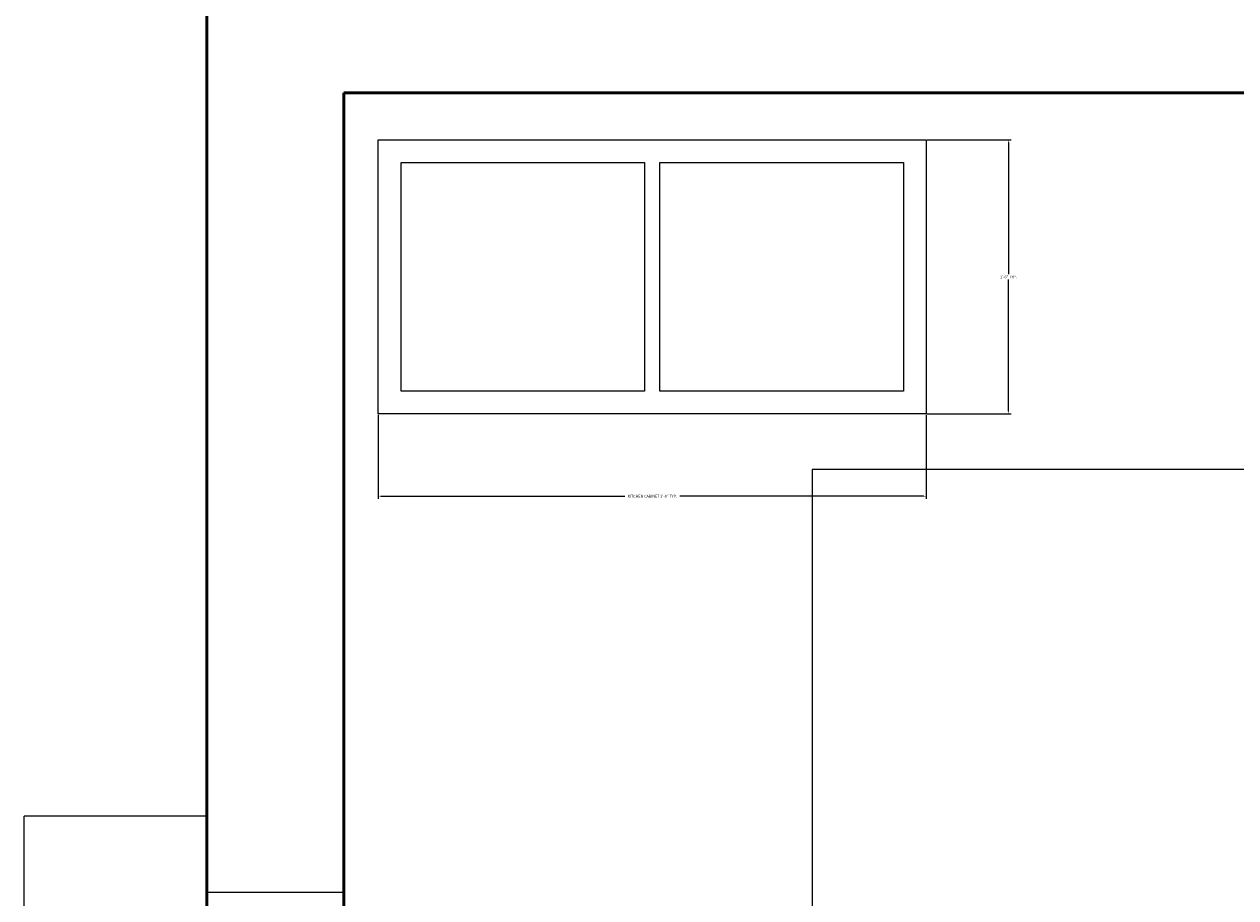
# Model space of a CAD drawing. Units: inches. Extents: x -105 to 1196, y -792 to 119.
# Tile 5 of 23: x -57 to 22, y -178 to -121. Entities that reach past the tile are written whole.
import ezdxf

# ---------------------------------------------------------------- set-up
doc = ezdxf.new("R2010")
doc.units = ezdxf.units.IN
doc.header["$MEASUREMENT"] = 0
for name, color, linetype, lineweight in [('A-ANNO-DIMS', 2, 'Continuous', 18), ('A-FLOR-FIXT', 8, 'Continuous', 18), ('A-GLAZ', 4, 'Continuous', 25), ('A-WALL', 3, 'Continuous', 50)]:
    doc.layers.add(name, color=color, linetype=linetype, lineweight=lineweight)
doc.styles.get("Standard").update_dxf_attribs({"font": 'arial.ttf'})
doc.dimstyles.get("Standard").update_dxf_attribs({"dimtxt": 0.18, "dimasz": 0.18, "dimexe": 0.18, "dimexo": 0.0625, "dimgap": 0.09, "dimtad": 0, "dimtih": 1, "dimtoh": 1, "dimdec": 1, "dimzin": 0, "dimdsep": 46, "dimlunit": 4, "dimtxsty": 'Standard', "dimcen": 0.09, "dimadec": 0, "dimazin": 0, "dimtfac": 1, "dimtdec": 1, "dimtofl": 0, "dimtmove": 0, "dimatfit": 3, "dimfxl": 1, "dimtolj": 1, "dimtzin": 0, "dimarcsym": 0})

# ---------------------------------------------------------------- blocks, each defined once
blk = doc.blocks.new('Wall Cabinet - 18 x 36 in front')
for p, q in [((17.5, -1.5), (17.5, -16.5)), ((18.5, -16.5), (18.5, -1.5))]:
    blk.add_line(p, q)
blk.add_lwpolyline([(0, -18), (0, 0), (36, 0), (36, -18)], close=True)
for points in [[(17.5, -16.5), (1.5, -16.5), (1.5, -1.5), (17.5, -1.5)], [(18.5, -1.5), (34.5, -1.5), (34.5, -16.5), (18.5, -16.5)]]:
    blk.add_lwpolyline(points)
blk = doc.blocks.new('WIN-1200')
at = {"ltscale": 2}
for p, q in [((12, 62), (0, 62)), ((0, 0), (0, 62)), ((12, 57), (12, 62)), ((12, 5), (12, 0)), ((12, 0), (0, 0))]:
    blk.add_line(p, q, dxfattribs=at)
for p, q in [((21, 57), (12, 57)), ((21, 5), (12, 5))]:
    blk.add_line(p, q)
blk = doc.blocks.new('*D69')
at = {"layer": 'A-ANNO-DIMS', "color": 0, "lineweight": -2, "transparency": 16777216}
for p, q in [((-33.991, -146.378), (-33.991, -151.895)), ((2.009, -146.378), (2.009, -151.895)), ((-33.811, -151.715), (-17.792, -151.715)), ((1.829, -151.715), (-14.19, -151.715))]:
    blk.add_line(p, q, dxfattribs=at)
at = {"layer": 'A-ANNO-DIMS', "color": 0, "transparency": 16777216}
for points in [[(-33.811, -151.685), (-33.811, -151.745), (-33.991, -151.715)], [(1.829, -151.685), (1.829, -151.745), (2.009, -151.715)]]:
    blk.add_solid(points, dxfattribs=at)
at = {"layer": 'Defpoints', "color": 0, "transparency": 16777216}
for p in [(-33.991, -146.315), (2.009, -146.315), (2.009, -151.715)]:
    blk.add_point(p, dxfattribs=at)
at = {"layer": 'A-ANNO-DIMS', "color": 0, "transparency": 16777216, "insert": (-15.991, -151.715), "char_height": 0.18, "attachment_point": 5}
blk.add_mtext('\\A1;KITCHEN CABINET 3\'-0" TYP.', dxfattribs=at)
blk = doc.blocks.new('*D70')
at = {"layer": 'A-ANNO-DIMS', "color": 0, "lineweight": -2, "transparency": 16777216}
for p, q in [((2.072, -128.315), (7.589, -128.315)), ((7.409, -128.495), (7.409, -137.133)), ((7.409, -146.135), (7.409, -137.497)), ((2.072, -146.315), (7.589, -146.315))]:
    blk.add_line(p, q, dxfattribs=at)
at = {"layer": 'A-ANNO-DIMS', "color": 0, "transparency": 16777216}
for points in [[(7.379, -128.495), (7.439, -128.495), (7.409, -128.315)], [(7.379, -146.135), (7.439, -146.135), (7.409, -146.315)]]:
    blk.add_solid(points, dxfattribs=at)
at = {"layer": 'Defpoints', "color": 0, "transparency": 16777216}
for p in [(2.009, -128.315), (7.409, -128.315), (2.009, -146.315)]:
    blk.add_point(p, dxfattribs=at)
at = {"layer": 'A-ANNO-DIMS', "color": 0, "transparency": 16777216, "insert": (7.409, -137.315), "char_height": 0.18, "attachment_point": 5}
blk.add_mtext('\\A1;1\'-6" TYP.', dxfattribs=at)

msp = doc.modelspace()

# ---------------------------------------------------------------- linework, layer by layer
at = {"layer": 'A-GLAZ'}
for p, q in [((120.744, -149.966), (-5.486, -149.966)), ((-5.486, -149.966), (-5.486, -282.227))]:
    msp.add_line(p, q, dxfattribs=at)
at = {"layer": 'A-WALL'}
for p, q in [((-45.256, 69.773), (-45.256, -125.227)), ((-45.256, -125.227), (-45.256, -291.227)), ((-36.256, -125.227), (120.744, -125.227)), ((-36.256, -125.227), (-36.256, -282.227))]:
    msp.add_line(p, q, dxfattribs=at)

# ---------------------------------------------------------------- block references
at = {"layer": 'A-FLOR-FIXT'}
msp.add_blockref('Wall Cabinet - 18 x 36 in front', (-33.991, -128.315), dxfattribs=at)
at = {"layer": 'A-GLAZ'}
msp.add_blockref('WIN-1200', (-57.256, -234.727), dxfattribs=at)

# ---------------------------------------------------------------- dimensions: what is measured, and where the dimension line sits
at = {"layer": 'A-ANNO-DIMS'}
dim = msp.add_linear_dim(base=(7.409, -128.315), p1=(2.009, -146.315), p2=(2.009, -128.315), angle=90, text='<> TYP.', dimstyle='Standard', override={"dimdec": 1, "dimlfac": 1, "dimrnd": 0, "dimzin": 1, "dimdsep": 46, "dimlunit": 4, "dimfrac": 2}, dxfattribs=at)
dim.commit()
dim.dimension.update_dxf_attribs({"geometry": '*D70', "text_midpoint": (7.409, -137.315)})
dim = msp.add_linear_dim(base=(2.009, -151.715), p1=(-33.991, -146.315), p2=(2.009, -146.315), text='KITCHEN CABINET <> TYP.', dimstyle='Standard', override={"dimdec": 1, "dimlfac": 1, "dimrnd": 0, "dimzin": 1, "dimdsep": 46, "dimlunit": 4, "dimfrac": 2}, dxfattribs=at)
dim.commit()
dim.dimension.update_dxf_attribs({"geometry": '*D69', "text_midpoint": (-15.991, -151.715)})

doc.saveas('drawing.dxf')
